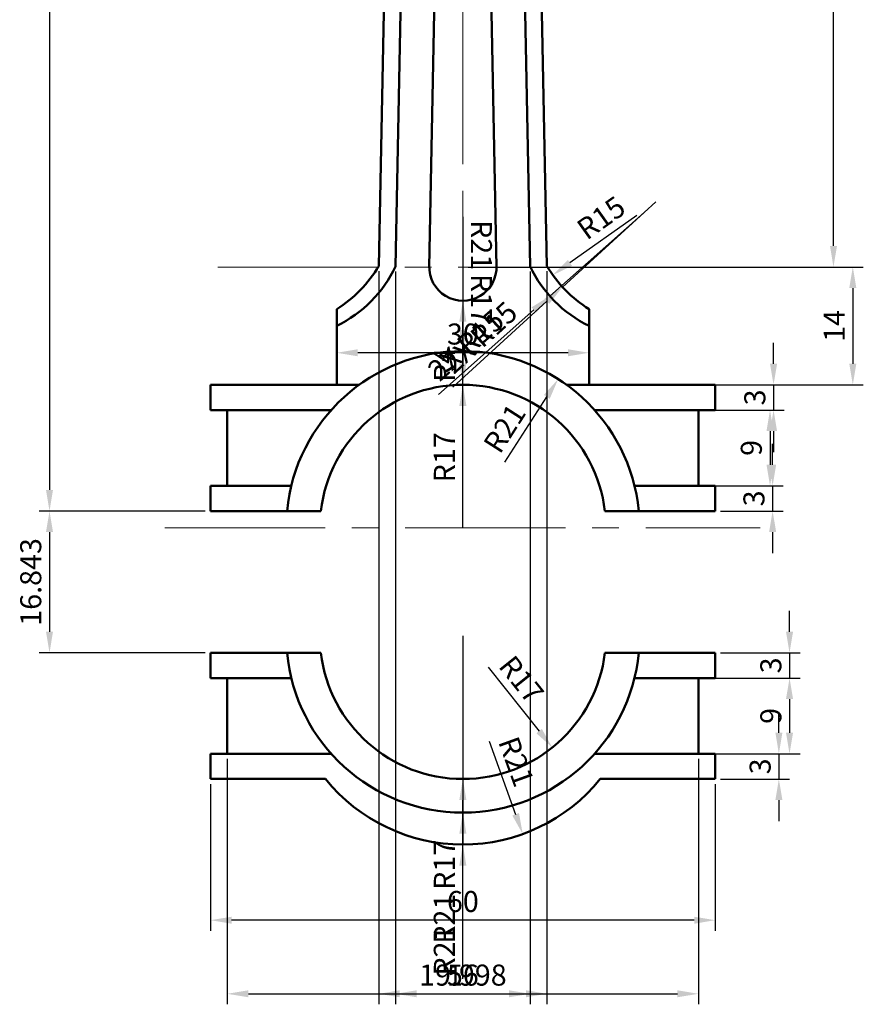
# Model space of a CAD drawing. Units: millimetres. Extents: x 2995 to 3180, y 2734 to 2968.
# Tile 1 of 3: x 2995 to 3095, y 2734 to 2851. Entities that reach past the tile are written whole.
import ezdxf

# ---------------------------------------------------------------- set-up
doc = ezdxf.new("R2010")
doc.units = ezdxf.units.MM
doc.linetypes.add('CENTER2', pattern=[28.575, 19.05, -3.175, 3.175, -3.175])
for name, color, linetype, lineweight in [('M-CNTR', 1, 'CENTER2', 18), ('M-DIMS', 2, 'Continuous', 25), ('M-OUTL', 7, 'Continuous', 50)]:
    doc.layers.add(name, color=color, linetype=linetype, lineweight=lineweight)
doc.styles.get("Standard").update_dxf_attribs({"font": 'arial.ttf'})
doc.dimstyles.new('ISO-25', dxfattribs={"dimtxt": 2.5, "dimasz": 2.5, "dimexe": 1.25, "dimexo": 0.625, "dimtad": 1, "dimtxsty": 'Standard', "dimcen": 2.5, "dimadec": 0, "dimazin": 0, "dimtfac": 1, "dimtmove": 0, "dimatfit": 3, "dimfxl": 1, "dimarcsym": 0})

# ---------------------------------------------------------------- blocks, each defined once
blk = doc.blocks.new('*D1')
at = {"layer": 'Defpoints', "color": 0, "transparency": 16777216}
for p in [(3047.54, 2807.77), (3047.54, 2790.77)]:
    blk.add_point(p, dxfattribs=at)
at = {"layer": 'M-DIMS', "color": 0, "lineweight": -2, "transparency": 16777216}
blk.add_line((3047.54, 2795.54), (3047.54, 2805.27), dxfattribs=at)
at = {"layer": 'M-DIMS', "color": 0, "transparency": 16777216}
blk.add_solid([(3047.12, 2805.27), (3047.96, 2805.27), (3047.54, 2807.77)], dxfattribs=at)
at = {"layer": 'M-DIMS', "color": 0, "transparency": 16777216, "insert": (3045.66, 2799.15), "char_height": 2.5, "attachment_point": 5, "rotation": 90}
blk.add_mtext('R17', dxfattribs=at)
blk = doc.blocks.new('*D2')
at = {"layer": 'Defpoints', "color": 0, "transparency": 16777216}
for p in [(3058.87, 2808.45), (3047.54, 2790.77)]:
    blk.add_point(p, dxfattribs=at)
at = {"layer": 'M-DIMS', "color": 0, "lineweight": -2, "transparency": 16777216}
blk.add_line((3052.53, 2798.56), (3057.52, 2806.35), dxfattribs=at)
at = {"layer": 'M-DIMS', "color": 0, "transparency": 16777216}
blk.add_solid([(3057.17, 2806.57), (3057.87, 2806.12), (3058.87, 2808.45)], dxfattribs=at)
at = {"layer": 'M-DIMS', "color": 0, "transparency": 16777216, "insert": (3052.77, 2802.42), "char_height": 2.5, "attachment_point": 5, "rotation": 57.3657}
blk.add_mtext('R21', dxfattribs=at)
blk = doc.blocks.new('*D3')
at = {"layer": 'Defpoints', "color": 0, "transparency": 16777216}
for p in [(3047.54, 2777.92), (3058.17, 2764.66)]:
    blk.add_point(p, dxfattribs=at)
at = {"layer": 'M-DIMS', "color": 0, "lineweight": -2, "transparency": 16777216}
blk.add_line((3050.53, 2774.2), (3056.61, 2766.61), dxfattribs=at)
at = {"layer": 'M-DIMS', "color": 0, "transparency": 16777216}
blk.add_solid([(3056.93, 2766.87), (3056.28, 2766.35), (3058.17, 2764.66)], dxfattribs=at)
at = {"layer": 'M-DIMS', "color": 0, "transparency": 16777216, "insert": (3054.25, 2772.55), "char_height": 2.5, "attachment_point": 5, "rotation": 308.7019}
blk.add_mtext('R17', dxfattribs=at)
blk = doc.blocks.new('*D4')
at = {"layer": 'Defpoints', "color": 0, "transparency": 16777216}
for p in [(3047.54, 2774.13), (3054.66, 2754.37)]:
    blk.add_point(p, dxfattribs=at)
at = {"layer": 'M-DIMS', "color": 0, "lineweight": -2, "transparency": 16777216}
blk.add_line((3050.68, 2765.42), (3053.81, 2756.72), dxfattribs=at)
at = {"layer": 'M-DIMS', "color": 0, "transparency": 16777216}
blk.add_solid([(3054.21, 2756.87), (3053.42, 2756.58), (3054.66, 2754.37)], dxfattribs=at)
at = {"layer": 'M-DIMS', "color": 0, "transparency": 16777216, "insert": (3053.59, 2762.88), "char_height": 2.5, "attachment_point": 5, "rotation": 289.8181}
blk.add_mtext('R21', dxfattribs=at)
blk = doc.blocks.new('*D5')
at = {"layer": 'Defpoints', "color": 0, "transparency": 16777216}
for p in [(3077.54, 2807.77), (3077.54, 2804.77), (3084.47, 2804.77)]:
    blk.add_point(p, dxfattribs=at)
at = {"layer": 'M-DIMS', "color": 0, "lineweight": -2, "transparency": 16777216}
for p, q in [((3084.47, 2810.27), (3084.47, 2812.77)), ((3078.17, 2807.77), (3085.72, 2807.77)), ((3084.47, 2807.77), (3084.47, 2804.77)), ((3078.17, 2804.77), (3085.72, 2804.77)), ((3084.47, 2802.27), (3084.47, 2799.77))]:
    blk.add_line(p, q, dxfattribs=at)
at = {"layer": 'M-DIMS', "color": 0, "transparency": 16777216}
for points in [[(3084.05, 2810.27), (3084.89, 2810.27), (3084.47, 2807.77)], [(3084.05, 2802.27), (3084.89, 2802.27), (3084.47, 2804.77)]]:
    blk.add_solid(points, dxfattribs=at)
at = {"layer": 'M-DIMS', "color": 0, "transparency": 16777216, "insert": (3082.57, 2806.27), "char_height": 2.5, "attachment_point": 5, "rotation": 90}
blk.add_mtext('3', dxfattribs=at)
blk = doc.blocks.new('*D6')
at = {"layer": 'Defpoints', "color": 0, "transparency": 16777216}
for p in [(3075.54, 2804.77), (3075.54, 2795.77), (3084.05, 2795.77)]:
    blk.add_point(p, dxfattribs=at)
at = {"layer": 'M-DIMS', "color": 0, "lineweight": -2, "transparency": 16777216}
for p, q in [((3076.17, 2804.77), (3085.3, 2804.77)), ((3084.05, 2802.27), (3084.05, 2798.27)), ((3076.17, 2795.77), (3085.3, 2795.77))]:
    blk.add_line(p, q, dxfattribs=at)
at = {"layer": 'M-DIMS', "color": 0, "transparency": 16777216}
for points in [[(3083.63, 2802.27), (3084.47, 2802.27), (3084.05, 2804.77)], [(3083.63, 2798.27), (3084.47, 2798.27), (3084.05, 2795.77)]]:
    blk.add_solid(points, dxfattribs=at)
at = {"layer": 'M-DIMS', "color": 0, "transparency": 16777216, "insert": (3082.15, 2800.27), "char_height": 2.5, "attachment_point": 5, "rotation": 90}
blk.add_mtext('9', dxfattribs=at)
blk = doc.blocks.new('*D7')
at = {"layer": 'Defpoints', "color": 0, "transparency": 16777216}
for p in [(3077.54, 2795.77), (3077.54, 2792.77), (3084.36, 2792.77)]:
    blk.add_point(p, dxfattribs=at)
at = {"layer": 'M-DIMS', "color": 0, "lineweight": -2, "transparency": 16777216}
for p, q in [((3084.36, 2798.27), (3084.36, 2800.77)), ((3078.17, 2795.77), (3085.61, 2795.77)), ((3084.36, 2795.77), (3084.36, 2792.77)), ((3078.17, 2792.77), (3085.61, 2792.77)), ((3084.36, 2790.27), (3084.36, 2787.77))]:
    blk.add_line(p, q, dxfattribs=at)
at = {"layer": 'M-DIMS', "color": 0, "transparency": 16777216}
for points in [[(3083.94, 2798.27), (3084.78, 2798.27), (3084.36, 2795.77)], [(3083.94, 2790.27), (3084.78, 2790.27), (3084.36, 2792.77)]]:
    blk.add_solid(points, dxfattribs=at)
at = {"layer": 'M-DIMS', "color": 0, "transparency": 16777216, "insert": (3082.46, 2794.27), "char_height": 2.5, "attachment_point": 5, "rotation": 90}
blk.add_mtext('3', dxfattribs=at)
blk = doc.blocks.new('*D8')
at = {"layer": 'Defpoints', "color": 0, "transparency": 16777216}
for p in [(3077.54, 2775.92), (3077.54, 2772.92), (3086.37, 2772.92)]:
    blk.add_point(p, dxfattribs=at)
at = {"layer": 'M-DIMS', "color": 0, "lineweight": -2, "transparency": 16777216}
for p, q in [((3086.37, 2778.42), (3086.37, 2780.92)), ((3078.17, 2775.92), (3087.62, 2775.92)), ((3086.37, 2775.92), (3086.37, 2772.92)), ((3078.17, 2772.92), (3087.62, 2772.92)), ((3086.37, 2770.42), (3086.37, 2767.92))]:
    blk.add_line(p, q, dxfattribs=at)
at = {"layer": 'M-DIMS', "color": 0, "transparency": 16777216}
for points in [[(3085.95, 2778.42), (3086.79, 2778.42), (3086.37, 2775.92)], [(3085.95, 2770.42), (3086.79, 2770.42), (3086.37, 2772.92)]]:
    blk.add_solid(points, dxfattribs=at)
at = {"layer": 'M-DIMS', "color": 0, "transparency": 16777216, "insert": (3084.47, 2774.42), "char_height": 2.5, "attachment_point": 5, "rotation": 90}
blk.add_mtext('3', dxfattribs=at)
blk = doc.blocks.new('*D9')
at = {"layer": 'Defpoints', "color": 0, "transparency": 16777216}
for p in [(3075.54, 2772.92), (3075.54, 2763.92), (3086.37, 2763.92)]:
    blk.add_point(p, dxfattribs=at)
at = {"layer": 'M-DIMS', "color": 0, "lineweight": -2, "transparency": 16777216}
for p, q in [((3076.17, 2772.92), (3087.62, 2772.92)), ((3086.37, 2770.42), (3086.37, 2766.42)), ((3076.17, 2763.92), (3087.62, 2763.92))]:
    blk.add_line(p, q, dxfattribs=at)
at = {"layer": 'M-DIMS', "color": 0, "transparency": 16777216}
for points in [[(3085.95, 2770.42), (3086.79, 2770.42), (3086.37, 2772.92)], [(3085.95, 2766.42), (3086.79, 2766.42), (3086.37, 2763.92)]]:
    blk.add_solid(points, dxfattribs=at)
at = {"layer": 'M-DIMS', "color": 0, "transparency": 16777216, "insert": (3084.47, 2768.42), "char_height": 2.5, "attachment_point": 5, "rotation": 90}
blk.add_mtext('9', dxfattribs=at)
blk = doc.blocks.new('*D10')
at = {"layer": 'Defpoints', "color": 0, "transparency": 16777216}
for p in [(3077.54, 2763.92), (3077.54, 2760.92), (3085.1, 2760.92)]:
    blk.add_point(p, dxfattribs=at)
at = {"layer": 'M-DIMS', "color": 0, "lineweight": -2, "transparency": 16777216}
for p, q in [((3085.1, 2766.42), (3085.1, 2768.92)), ((3078.17, 2763.92), (3086.35, 2763.92)), ((3085.1, 2763.92), (3085.1, 2760.92)), ((3078.17, 2760.92), (3086.35, 2760.92)), ((3085.1, 2758.42), (3085.1, 2755.92))]:
    blk.add_line(p, q, dxfattribs=at)
at = {"layer": 'M-DIMS', "color": 0, "transparency": 16777216}
for points in [[(3084.69, 2766.42), (3085.52, 2766.42), (3085.1, 2763.92)], [(3084.69, 2758.42), (3085.52, 2758.42), (3085.1, 2760.92)]]:
    blk.add_solid(points, dxfattribs=at)
at = {"layer": 'M-DIMS', "color": 0, "transparency": 16777216, "insert": (3083.2, 2762.42), "char_height": 2.5, "attachment_point": 5, "rotation": 90}
blk.add_mtext('3', dxfattribs=at)
blk = doc.blocks.new('*D11')
at = {"layer": 'Defpoints', "color": 0, "transparency": 16777216}
for p in [(3017.54, 2760.92), (3077.54, 2760.92), (3017.54, 2744.14)]:
    blk.add_point(p, dxfattribs=at)
at = {"layer": 'M-DIMS', "color": 0, "lineweight": -2, "transparency": 16777216}
for p, q in [((3017.54, 2760.3), (3017.54, 2742.89)), ((3077.54, 2760.3), (3077.54, 2742.89)), ((3075.04, 2744.14), (3020.04, 2744.14))]:
    blk.add_line(p, q, dxfattribs=at)
at = {"layer": 'M-DIMS', "color": 0, "transparency": 16777216}
for points in [[(3020.04, 2744.55), (3020.04, 2743.72), (3017.54, 2744.14)], [(3075.04, 2744.55), (3075.04, 2743.72), (3077.54, 2744.14)]]:
    blk.add_solid(points, dxfattribs=at)
at = {"layer": 'M-DIMS', "color": 0, "transparency": 16777216, "insert": (3047.54, 2746.04), "char_height": 2.5, "attachment_point": 5}
blk.add_mtext('60', dxfattribs=at)
blk = doc.blocks.new('*D12')
at = {"layer": 'Defpoints', "color": 0, "transparency": 16777216}
for p in [(3032.54, 2816.77), (3062.54, 2816.77), (3032.54, 2811.58)]:
    blk.add_point(p, dxfattribs=at)
at = {"layer": 'M-DIMS', "color": 0, "lineweight": -2, "transparency": 16777216}
for p, q in [((3032.54, 2816.14), (3032.54, 2810.33)), ((3062.54, 2816.14), (3062.54, 2810.33)), ((3060.04, 2811.58), (3035.04, 2811.58))]:
    blk.add_line(p, q, dxfattribs=at)
at = {"layer": 'M-DIMS', "color": 0, "transparency": 16777216}
for points in [[(3035.04, 2811.99), (3035.04, 2811.16), (3032.54, 2811.58)], [(3060.04, 2811.99), (3060.04, 2811.16), (3062.54, 2811.58)]]:
    blk.add_solid(points, dxfattribs=at)
at = {"layer": 'M-DIMS', "color": 0, "transparency": 16777216, "insert": (3047.54, 2813.48), "char_height": 2.5, "attachment_point": 5}
blk.add_mtext('30', dxfattribs=at)
blk = doc.blocks.new('*D13')
at = {"layer": 'Defpoints', "color": 0, "transparency": 16777216}
for p in [(3070.46, 2829.5), (3058.24, 2820.81)]:
    blk.add_point(p, dxfattribs=at)
at = {"layer": 'M-DIMS', "color": 0, "lineweight": -2, "transparency": 16777216}
blk.add_line((3068.21, 2827.91), (3060.27, 2822.26), dxfattribs=at)
at = {"layer": 'M-DIMS', "color": 0, "transparency": 16777216}
blk.add_solid([(3060.03, 2822.6), (3060.52, 2821.92), (3058.24, 2820.81)], dxfattribs=at)
at = {"layer": 'M-DIMS', "color": 0, "transparency": 16777216, "insert": (3064.16, 2827.36), "char_height": 2.5, "attachment_point": 5, "rotation": 35.4212}
blk.add_mtext('R15', dxfattribs=at)
blk = doc.blocks.new('*D14')
at = {"layer": 'Defpoints', "color": 0, "transparency": 16777216}
for p in [(3047.54, 2821.77), (3062.54, 2807.77), (3093.89, 2807.77)]:
    blk.add_point(p, dxfattribs=at)
at = {"layer": 'M-DIMS', "color": 0, "lineweight": -2, "transparency": 16777216}
for p, q in [((3048.17, 2821.77), (3095.14, 2821.77)), ((3093.89, 2819.27), (3093.89, 2810.27)), ((3063.17, 2807.77), (3095.14, 2807.77))]:
    blk.add_line(p, q, dxfattribs=at)
at = {"layer": 'M-DIMS', "color": 0, "transparency": 16777216}
for points in [[(3093.47, 2819.27), (3094.31, 2819.27), (3093.89, 2821.77)], [(3093.47, 2810.27), (3094.31, 2810.27), (3093.89, 2807.77)]]:
    blk.add_solid(points, dxfattribs=at)
at = {"layer": 'M-DIMS', "color": 0, "transparency": 16777216, "insert": (3092.01, 2814.77), "char_height": 2.5, "attachment_point": 5, "rotation": 90}
blk.add_mtext('14', dxfattribs=at)
blk = doc.blocks.new('*D15')
at = {"layer": 'Defpoints', "color": 0, "transparency": 16777216}
for p in [(3049.54, 2921.77), (3091.59, 2921.77), (3047.54, 2821.77)]:
    blk.add_point(p, dxfattribs=at)
at = {"layer": 'M-DIMS', "color": 0, "lineweight": -2, "transparency": 16777216}
for p, q in [((3050.17, 2921.77), (3092.84, 2921.77)), ((3091.59, 2824.27), (3091.59, 2919.27)), ((3048.17, 2821.77), (3092.84, 2821.77))]:
    blk.add_line(p, q, dxfattribs=at)
at = {"layer": 'M-DIMS', "color": 0, "transparency": 16777216}
for points in [[(3091.18, 2919.27), (3092.01, 2919.27), (3091.59, 2921.77)], [(3091.18, 2824.27), (3092.01, 2824.27), (3091.59, 2821.77)]]:
    blk.add_solid(points, dxfattribs=at)
at = {"layer": 'M-DIMS', "color": 0, "transparency": 16777216, "insert": (3089.69, 2871.77), "char_height": 2.5, "attachment_point": 5, "rotation": 90}
blk.add_mtext('100', dxfattribs=at)
blk = doc.blocks.new('*D28')
at = {"layer": 'Defpoints', "color": 0, "transparency": 16777216}
for p in [(3047.54, 2953.77), (2998.41, 2792.77), (3017.54, 2792.77)]:
    blk.add_point(p, dxfattribs=at)
at = {"layer": 'M-DIMS', "color": 0, "lineweight": -2, "transparency": 16777216}
for p, q in [((3046.92, 2953.77), (2997.16, 2953.77)), ((2998.41, 2951.27), (2998.41, 2795.27)), ((3016.92, 2792.77), (2997.16, 2792.77))]:
    blk.add_line(p, q, dxfattribs=at)
at = {"layer": 'M-DIMS', "color": 0, "transparency": 16777216}
for points in [[(2997.99, 2951.27), (2998.82, 2951.27), (2998.41, 2953.77)], [(2997.99, 2795.27), (2998.82, 2795.27), (2998.41, 2792.77)]]:
    blk.add_solid(points, dxfattribs=at)
at = {"layer": 'M-DIMS', "color": 0, "transparency": 16777216, "insert": (2996.5, 2873.27), "char_height": 2.5, "attachment_point": 5, "rotation": 90}
blk.add_mtext('161', dxfattribs=at)
blk = doc.blocks.new('*D29')
at = {"layer": 'Defpoints', "color": 0, "transparency": 16777216}
for p in [(3017.54, 2792.77), (2998.41, 2775.92), (3017.54, 2775.92)]:
    blk.add_point(p, dxfattribs=at)
at = {"layer": 'M-DIMS', "color": 0, "lineweight": -2, "transparency": 16777216}
for p, q in [((3016.92, 2792.77), (2997.16, 2792.77)), ((2998.41, 2790.27), (2998.41, 2778.42)), ((3016.92, 2775.92), (2997.16, 2775.92))]:
    blk.add_line(p, q, dxfattribs=at)
at = {"layer": 'M-DIMS', "color": 0, "transparency": 16777216}
for points in [[(2997.99, 2790.27), (2998.82, 2790.27), (2998.41, 2792.77)], [(2997.99, 2778.42), (2998.82, 2778.42), (2998.41, 2775.92)]]:
    blk.add_solid(points, dxfattribs=at)
at = {"layer": 'M-DIMS', "color": 0, "transparency": 16777216, "insert": (2996.5, 2784.34), "char_height": 2.5, "attachment_point": 5, "rotation": 90}
blk.add_mtext('16.843', dxfattribs=at)
blk = doc.blocks.new('*D32')
at = {"layer": 'Defpoints', "color": 0, "transparency": 16777216}
for p in [(3039.54, 2821.85), (3055.54, 2821.85), (3055.54, 2735.39)]:
    blk.add_point(p, dxfattribs=at)
at = {"layer": 'M-DIMS', "color": 0, "lineweight": -2, "transparency": 16777216}
for p, q in [((3039.54, 2821.22), (3039.54, 2734.14)), ((3055.54, 2821.22), (3055.54, 2734.14)), ((3042.04, 2735.39), (3053.04, 2735.39))]:
    blk.add_line(p, q, dxfattribs=at)
at = {"layer": 'M-DIMS', "color": 0, "transparency": 16777216}
for points in [[(3042.04, 2735.81), (3042.04, 2734.98), (3039.54, 2735.39)], [(3053.04, 2735.81), (3053.04, 2734.98), (3055.54, 2735.39)]]:
    blk.add_solid(points, dxfattribs=at)
at = {"layer": 'M-DIMS', "color": 0, "transparency": 16777216, "insert": (3047.54, 2737.29), "char_height": 2.5, "attachment_point": 5}
blk.add_mtext('16', dxfattribs=at)
blk = doc.blocks.new('*D33')
at = {"layer": 'Defpoints', "color": 0, "transparency": 16777216}
for p in [(3037.54, 2821.89), (3057.54, 2821.89), (3057.54, 2735.39)]:
    blk.add_point(p, dxfattribs=at)
at = {"layer": 'M-DIMS', "color": 0, "lineweight": -2, "transparency": 16777216}
for p, q in [((3037.54, 2821.26), (3037.54, 2734.14)), ((3057.54, 2821.26), (3057.54, 2734.14)), ((3040.04, 2735.39), (3055.04, 2735.39))]:
    blk.add_line(p, q, dxfattribs=at)
at = {"layer": 'M-DIMS', "color": 0, "transparency": 16777216}
for points in [[(3040.04, 2735.81), (3040.04, 2734.98), (3037.54, 2735.39)], [(3055.04, 2735.81), (3055.04, 2734.98), (3057.54, 2735.39)]]:
    blk.add_solid(points, dxfattribs=at)
at = {"layer": 'M-DIMS', "color": 0, "transparency": 16777216, "insert": (3047.54, 2737.29), "char_height": 2.5, "attachment_point": 5}
blk.add_mtext('19.998', dxfattribs=at)
blk = doc.blocks.new('*D34')
at = {"layer": 'Defpoints', "color": 0, "transparency": 16777216}
for p in [(3019.54, 2763.92), (3075.54, 2763.92), (3075.54, 2735.39)]:
    blk.add_point(p, dxfattribs=at)
at = {"layer": 'M-DIMS', "color": 0, "lineweight": -2, "transparency": 16777216}
for p, q in [((3019.54, 2763.3), (3019.54, 2734.14)), ((3075.54, 2763.3), (3075.54, 2734.14)), ((3022.04, 2735.39), (3073.04, 2735.39))]:
    blk.add_line(p, q, dxfattribs=at)
at = {"layer": 'M-DIMS', "color": 0, "transparency": 16777216}
for points in [[(3022.04, 2735.81), (3022.04, 2734.98), (3019.54, 2735.39)], [(3073.04, 2735.81), (3073.04, 2734.98), (3075.54, 2735.39)]]:
    blk.add_solid(points, dxfattribs=at)
at = {"layer": 'M-DIMS', "color": 0, "transparency": 16777216, "insert": (3047.54, 2737.29), "char_height": 2.5, "attachment_point": 5}
blk.add_mtext('56', dxfattribs=at)
blk = doc.blocks.new('*D43')
at = {"layer": 'Defpoints', "color": 0, "transparency": 16777216}
for p in [(3047.54, 2821.77), (3047.54, 2817.77)]:
    blk.add_point(p, dxfattribs=at)
at = {"layer": 'M-DIMS', "color": 0, "lineweight": -2, "transparency": 16777216}
for p, q in [((3047.54, 2821.77), (3047.54, 2817.77)), ((3047.54, 2807.5), (3047.54, 2815.27))]:
    blk.add_line(p, q, dxfattribs=at)
at = {"layer": 'M-DIMS', "color": 0, "transparency": 16777216}
blk.add_solid([(3047.12, 2815.27), (3047.96, 2815.27), (3047.54, 2817.77)], dxfattribs=at)
at = {"layer": 'M-DIMS', "color": 0, "transparency": 16777216, "insert": (3045.67, 2810.13), "char_height": 2.5, "attachment_point": 5, "rotation": 89.9963}
blk.add_mtext('R4', dxfattribs=at)
blk = doc.blocks.new('*D44')
at = {"layer": 'Defpoints', "color": 0, "transparency": 16777216}
for p in [(3070.46, 2829.5), (3059.38, 2819.39)]:
    blk.add_point(p, dxfattribs=at)
at = {"layer": 'M-DIMS', "color": 0, "lineweight": -2, "transparency": 16777216}
for p, q in [((3070.46, 2829.5), (3059.38, 2819.39)), ((3046.34, 2807.49), (3057.54, 2817.71))]:
    blk.add_line(p, q, dxfattribs=at)
at = {"layer": 'M-DIMS', "color": 0, "transparency": 16777216}
blk.add_solid([(3057.25, 2818.01), (3057.82, 2817.4), (3059.38, 2819.39)], dxfattribs=at)
at = {"layer": 'M-DIMS', "color": 0, "transparency": 16777216, "insert": (3049.73, 2813.16), "char_height": 2.5, "attachment_point": 5, "rotation": 42.3887}
blk.add_mtext('2X R15', dxfattribs=at)
blk = doc.blocks.new('*D45')
at = {"layer": 'Defpoints', "color": 0, "transparency": 16777216}
for p in [(3069.1, 2828.26), (3057.86, 2818.32)]:
    blk.add_point(p, dxfattribs=at)
at = {"layer": 'M-DIMS', "color": 0, "lineweight": -2, "transparency": 16777216}
for p, q in [((3069.1, 2828.26), (3057.86, 2818.32)), ((3044.63, 2806.63), (3055.99, 2816.67))]:
    blk.add_line(p, q, dxfattribs=at)
at = {"layer": 'M-DIMS', "color": 0, "transparency": 16777216}
blk.add_solid([(3055.71, 2816.98), (3056.27, 2816.35), (3057.86, 2818.32)], dxfattribs=at)
at = {"layer": 'M-DIMS', "color": 0, "transparency": 16777216, "insert": (3048.12, 2812.24), "char_height": 2.5, "attachment_point": 5, "rotation": 41.473}
blk.add_mtext('2X R15', dxfattribs=at)
blk = doc.blocks.new('*D46')
at = {"layer": 'Defpoints', "color": 0, "transparency": 16777216}
for p in [(3047.54, 2811.77), (3047.54, 2790.77)]:
    blk.add_point(p, dxfattribs=at)
at = {"layer": 'M-DIMS', "color": 0, "lineweight": -2, "transparency": 16777216}
for p, q in [((3047.54, 2827.74), (3047.54, 2814.27)), ((3047.54, 2790.77), (3047.54, 2811.77))]:
    blk.add_line(p, q, dxfattribs=at)
at = {"layer": 'M-DIMS', "color": 0, "transparency": 16777216}
blk.add_solid([(3047.96, 2814.27), (3047.12, 2814.27), (3047.54, 2811.77)], dxfattribs=at)
at = {"layer": 'M-DIMS', "color": 0, "transparency": 16777216, "insert": (3049.42, 2824.37), "char_height": 2.5, "attachment_point": 5, "rotation": 270.0007}
blk.add_mtext('R21', dxfattribs=at)
blk = doc.blocks.new('*D47')
at = {"layer": 'Defpoints', "color": 0, "transparency": 16777216}
for p in [(3047.54, 2807.77), (3047.54, 2790.77)]:
    blk.add_point(p, dxfattribs=at)
at = {"layer": 'M-DIMS', "color": 0, "lineweight": -2, "transparency": 16777216}
for p, q in [((3047.54, 2821.58), (3047.54, 2810.27)), ((3047.54, 2790.77), (3047.54, 2807.77))]:
    blk.add_line(p, q, dxfattribs=at)
at = {"layer": 'M-DIMS', "color": 0, "transparency": 16777216}
blk.add_solid([(3047.96, 2810.27), (3047.12, 2810.27), (3047.54, 2807.77)], dxfattribs=at)
at = {"layer": 'M-DIMS', "color": 0, "transparency": 16777216, "insert": (3049.42, 2817.97), "char_height": 2.5, "attachment_point": 5, "rotation": 270.0009}
blk.add_mtext('R17', dxfattribs=at)
blk = doc.blocks.new('*D48')
at = {"layer": 'Defpoints', "color": 0, "transparency": 16777216}
for p in [(3047.54, 2777.92), (3047.54, 2760.92)]:
    blk.add_point(p, dxfattribs=at)
at = {"layer": 'M-DIMS', "color": 0, "lineweight": -2, "transparency": 16777216}
for p, q in [((3047.54, 2777.92), (3047.54, 2760.92)), ((3047.54, 2747.11), (3047.54, 2758.42))]:
    blk.add_line(p, q, dxfattribs=at)
at = {"layer": 'M-DIMS', "color": 0, "transparency": 16777216}
blk.add_solid([(3047.12, 2758.42), (3047.96, 2758.42), (3047.54, 2760.92)], dxfattribs=at)
at = {"layer": 'M-DIMS', "color": 0, "transparency": 16777216, "insert": (3045.66, 2750.72), "char_height": 2.5, "attachment_point": 5, "rotation": 89.9991}
blk.add_mtext('R17', dxfattribs=at)
blk = doc.blocks.new('*D49')
at = {"layer": 'Defpoints', "color": 0, "transparency": 16777216}
for p in [(3047.54, 2777.92), (3047.54, 2756.92)]:
    blk.add_point(p, dxfattribs=at)
at = {"layer": 'M-DIMS', "color": 0, "lineweight": -2, "transparency": 16777216}
for p, q in [((3047.54, 2777.92), (3047.54, 2756.92)), ((3047.54, 2740.95), (3047.54, 2754.42))]:
    blk.add_line(p, q, dxfattribs=at)
at = {"layer": 'M-DIMS', "color": 0, "transparency": 16777216}
blk.add_solid([(3047.12, 2754.42), (3047.96, 2754.42), (3047.54, 2756.92)], dxfattribs=at)
at = {"layer": 'M-DIMS', "color": 0, "transparency": 16777216, "insert": (3045.66, 2744.32), "char_height": 2.5, "attachment_point": 5, "rotation": 89.9993}
blk.add_mtext('R21', dxfattribs=at)
blk = doc.blocks.new('*D50')
at = {"layer": 'Defpoints', "color": 0, "transparency": 16777216}
for p in [(3047.54, 2774.13), (3047.54, 2753.13)]:
    blk.add_point(p, dxfattribs=at)
at = {"layer": 'M-DIMS', "color": 0, "lineweight": -2, "transparency": 16777216}
for p, q in [((3047.54, 2774.13), (3047.54, 2753.13)), ((3047.54, 2737.16), (3047.54, 2750.63))]:
    blk.add_line(p, q, dxfattribs=at)
at = {"layer": 'M-DIMS', "color": 0, "transparency": 16777216}
blk.add_solid([(3047.12, 2750.63), (3047.96, 2750.63), (3047.54, 2753.13)], dxfattribs=at)
at = {"layer": 'M-DIMS', "color": 0, "transparency": 16777216, "insert": (3045.66, 2740.53), "char_height": 2.5, "attachment_point": 5, "rotation": 89.9993}
blk.add_mtext('R21', dxfattribs=at)

msp = doc.modelspace()

# ---------------------------------------------------------------- linework, layer by layer
at = {"layer": 'M-CNTR'}
for p, q in [((3047.5413, 2938.7662), (3047.5413, 2821.7662)), ((3018.4256, 2821.7662), (3087.998, 2821.7662)), ((3047.5413, 2821.7662), (3047.5413, 2814.7662)), ((3047.5413, 2807.7662), (3047.5413, 2790.7662)), ((3012.1191, 2790.7662), (3082.8947, 2790.7662)), ((3047.5413, 2760.9236), (3047.5413, 2777.9236))]:
    msp.add_line(p, q, dxfattribs=at)
at = {"layer": 'M-OUTL'}
for p, q in [((3041.5351, 2921.4996), (3039.5421, 2821.8462)), ((3045.5413, 2921.7662), (3043.5413, 2821.7662)), ((3049.5413, 2921.7662), (3051.5413, 2821.7662)), ((3053.5474, 2921.4996), (3055.5405, 2821.8462)), ((3039.49, 2919.2627), (3037.5425, 2821.8862)), ((3055.5925, 2919.2627), (3057.5401, 2821.8862)), ((3032.5413, 2814.7662), (3032.5413, 2816.7662)), ((3062.5413, 2814.7662), (3062.5413, 2816.7662)), ((3032.5413, 2814.7662), (3032.5413, 2807.7662)), ((3062.5413, 2814.7662), (3062.5413, 2807.7662)), ((3017.5413, 2804.7662), (3017.5413, 2807.7662)), ((3017.5413, 2807.7662), (3032.5413, 2807.7662)), ((3035.2124, 2807.7662), (3032.5413, 2807.7662)), ((3062.5413, 2807.7662), (3059.8701, 2807.7662)), ((3062.5413, 2807.7662), (3077.5413, 2807.7662)), ((3077.5413, 2807.7662), (3077.5413, 2804.7662)), ((3031.8888, 2804.7662), (3017.5413, 2804.7662)), ((3019.5413, 2804.7662), (3017.5413, 2804.7662)), ((3019.5413, 2795.7662), (3019.5413, 2804.7662)), ((3077.5413, 2804.7662), (3063.1937, 2804.7662)), ((3077.5413, 2804.7662), (3075.5413, 2804.7662)), ((3075.5413, 2804.7662), (3075.5413, 2795.7662)), ((3017.5413, 2792.7662), (3017.5413, 2795.7662)), ((3017.5413, 2795.7662), (3019.5413, 2795.7662)), ((3027.1452, 2795.7662), (3019.5413, 2795.7662)), ((3075.5413, 2795.7662), (3067.9373, 2795.7662)), ((3075.5413, 2795.7662), (3077.5413, 2795.7662)), ((3077.5413, 2795.7662), (3077.5413, 2792.7662)), ((3026.6367, 2792.7662), (3017.5413, 2792.7662)), ((3026.6367, 2792.7662), (3030.6593, 2792.7662)), ((3064.4232, 2792.7662), (3068.4458, 2792.7662)), ((3077.5413, 2792.7662), (3068.4458, 2792.7662)), ((3017.5413, 2772.9236), (3017.5413, 2775.9236)), ((3017.5413, 2775.9236), (3026.6367, 2775.9236)), ((3030.6593, 2775.9236), (3026.6367, 2775.9236)), ((3068.4458, 2775.9236), (3064.4232, 2775.9236)), ((3068.4458, 2775.9236), (3077.5413, 2775.9236)), ((3077.5413, 2775.9236), (3077.5413, 2772.9236)), ((3019.5413, 2772.9236), (3017.5413, 2772.9236)), ((3019.5413, 2763.9236), (3019.5413, 2772.9236)), ((3019.5413, 2772.9236), (3027.1452, 2772.9236)), ((3067.9373, 2772.9236), (3075.5413, 2772.9236)), ((3075.5413, 2772.9236), (3075.5413, 2763.9236)), ((3077.5413, 2772.9236), (3075.5413, 2772.9236)), ((3017.5413, 2760.9236), (3017.5413, 2763.9236)), ((3017.5413, 2763.9236), (3031.8888, 2763.9236)), ((3017.5413, 2763.9236), (3019.5413, 2763.9236)), ((3063.1937, 2763.9236), (3077.5413, 2763.9236)), ((3075.5413, 2763.9236), (3077.5413, 2763.9236)), ((3077.5413, 2763.9236), (3077.5413, 2760.9236)), ((3031.2124, 2760.9236), (3017.5413, 2760.9236)), ((3077.5413, 2760.9236), (3063.8701, 2760.9236))]:
    msp.add_line(p, q, dxfattribs=at)
for centre, radius, start, end in [((3024.6214, 2829.5049), 15, 301.869919, 329.4748), ((3025.9802, 2828.2552), 15, 295.93852, 334.705886), ((3047.5413, 2821.7662), 4, 177.708474, 2.291526), ((3069.1024, 2828.2552), 15, 205.294114, 244.06148), ((3070.4611, 2829.5049), 15, 210.5252, 238.130081), ((3047.5413, 2790.7662), 21, 5.465024, 174.534976), ((3047.5413, 2790.7662), 17, 6.756327, 173.243673), ((3047.5413, 2777.9236), 21, 185.465024, 354.534976), ((3047.5413, 2777.9236), 17, 186.756327, 353.243673), ((3047.5413, 2774.1285), 21, 218.961994, 321.038006)]:
    msp.add_arc(centre, radius, start, end, dxfattribs=at)

# ---------------------------------------------------------------- dimensions: what is measured, and where the dimension line sits
at = {"layer": 'M-DIMS'}
for base, p1, p2, override, picture, middle in [((2998.4052, 2792.7662), (3047.5413, 2953.7662), (3017.5413, 2792.7662), {"dimdec": 0, "dimlfac": 1, "dimrnd": 0, "dimzin": 0, "dimdsep": 46, "dimlunit": 2}, '*D28', (2996.5038, 2873.2662)), ((3091.5923, 2921.7662), (3047.5413, 2821.7662), (3049.5413, 2921.7662), {"dimclrd": 0, "dimclre": 0, "dimclrt": 0}, '*D15', (3089.6908, 2871.7662)), ((3093.8887, 2807.7662), (3047.5413, 2821.7662), (3062.5413, 2807.7662), {"dimclrd": 0, "dimclre": 0, "dimclrt": 0}, '*D14', (3092.0086, 2814.7662)), ((3084.4716, 2804.7662), (3077.5413, 2807.7662), (3077.5413, 2804.7662), {"dimclrd": 0, "dimclre": 0, "dimclrt": 0}, '*D5', (3082.5693, 2806.2662)), ((3084.0497, 2795.7662), (3075.5413, 2804.7662), (3075.5413, 2795.7662), {"dimclrd": 0, "dimclre": 0, "dimclrt": 0}, '*D6', (3082.1483, 2800.2662)), ((3084.3603, 2792.7662), (3077.5413, 2795.7662), (3077.5413, 2792.7662), {"dimclrd": 0, "dimclre": 0, "dimclrt": 0}, '*D7', (3082.458, 2794.2662)), ((2998.4052, 2775.9236), (3017.5413, 2792.7662), (3017.5413, 2775.9236), {"dimdec": 3, "dimlfac": 1, "dimrnd": 0, "dimzin": 0, "dimdsep": 46, "dimlunit": 2}, '*D29', (2996.5029, 2784.3449)), ((3086.3701, 2772.9236), (3077.5413, 2775.9236), (3077.5413, 2772.9236), {"dimclrd": 0, "dimclre": 0, "dimclrt": 0}, '*D8', (3084.4678, 2774.4236)), ((3086.3701, 2763.9236), (3075.5413, 2772.9236), (3075.5413, 2763.9236), {"dimclrd": 0, "dimclre": 0, "dimclrt": 0}, '*D9', (3084.4686, 2768.4236)), ((3085.1044, 2760.9236), (3077.5413, 2763.9236), (3077.5413, 2760.9236), {"dimclrd": 0, "dimclre": 0, "dimclrt": 0}, '*D10', (3083.2021, 2762.4236))]:
    dim = msp.add_linear_dim(base=base, p1=p1, p2=p2, angle=90, dimstyle='ISO-25', override=override, dxfattribs=at)
    dim.commit()
    dim.dimension.update_dxf_attribs({"geometry": picture, "text_midpoint": middle})
for center, mpoint, override, picture, middle in [((3070.4611, 2829.5049), (3058.2374, 2820.8112), {"dimclrd": 0, "dimclre": 0, "dimclrt": 0}, '*D13', (3065.263, 2825.8079)), ((3047.5413, 2790.7662), (3047.541, 2811.7662), {"dimdec": 0, "dimlfac": 1, "dimrnd": 0, "dimzin": 0, "dimdsep": 46, "dimlunit": 2}, '*D46', (3047.5408, 2824.3662)), ((3047.5413, 2790.7662), (3047.541, 2807.7662), {"dimdec": 0, "dimlfac": 1, "dimrnd": 0, "dimzin": 0, "dimdsep": 46, "dimlunit": 2}, '*D47', (3047.5408, 2817.9662)), ((3047.5413, 2790.7662), (3047.5413, 2807.7662), {"dimclrd": 0, "dimclre": 0, "dimclrt": 0}, '*D1', (3047.5413, 2799.1543)), ((3047.5413, 2790.7662), (3058.866, 2808.4509), {"dimclrd": 0, "dimclre": 0, "dimclrt": 0}, '*D2', (3054.352, 2801.4018)), ((3047.5413, 2777.9236), (3047.541, 2760.9236), {"dimdec": 0, "dimlfac": 1, "dimrnd": 0, "dimzin": 0, "dimdsep": 46, "dimlunit": 2}, '*D48', (3047.5408, 2750.7236)), ((3047.5413, 2777.9236), (3047.541, 2756.9236), {"dimdec": 0, "dimlfac": 1, "dimrnd": 0, "dimzin": 0, "dimdsep": 46, "dimlunit": 2}, '*D49', (3047.5408, 2744.3236)), ((3047.5413, 2777.9236), (3058.1708, 2764.6567), {"dimclrd": 0, "dimclre": 0, "dimclrt": 0}, '*D3', (3052.7861, 2771.3774)), ((3047.5413, 2774.1285), (3047.541, 2753.1285), {"dimdec": 0, "dimlfac": 1, "dimrnd": 0, "dimzin": 0, "dimdsep": 46, "dimlunit": 2}, '*D50', (3047.5408, 2740.5285)), ((3047.5413, 2774.1285), (3054.661, 2754.3723), {"dimclrd": 0, "dimclre": 0, "dimclrt": 0}, '*D4', (3051.8231, 2762.2471))]:
    dim = msp.add_radius_dim(center=center, mpoint=mpoint, dimstyle='ISO-25', override=override, dxfattribs=at)
    dim.commit()
    dim.dimension.update_dxf_attribs({"geometry": picture, "text_midpoint": middle, "dimtype": 164})
for center, mpoint, picture, middle in [((3070.4611, 2829.5049), (3059.3823, 2819.3926), '*D44', (3049.7334, 2813.1598)), ((3069.1024, 2828.2552), (3057.8633, 2818.3211), '*D45', (3048.116, 2812.2434))]:
    dim = msp.add_radius_dim(center=center, mpoint=mpoint, text='2X <>', dimstyle='ISO-25', override={"dimdec": 0, "dimlfac": 1, "dimrnd": 0, "dimzin": 0, "dimdsep": 46, "dimlunit": 2}, dxfattribs=at)
    dim.commit()
    dim.dimension.update_dxf_attribs({"geometry": picture, "text_midpoint": middle})
for base, p1, p2, override, picture, middle in [((3057.5401, 2735.3926), (3037.5425, 2821.8862), (3057.5401, 2821.8862), {"dimdec": 3, "dimlfac": 1, "dimrnd": 0, "dimzin": 0, "dimdsep": 46, "dimlunit": 2}, '*D33', (3047.5413, 2737.2941)), ((3055.5405, 2735.3926), (3039.5421, 2821.8462), (3055.5405, 2821.8462), {"dimdec": 0, "dimlfac": 1, "dimrnd": 0, "dimzin": 0, "dimdsep": 46, "dimlunit": 2}, '*D32', (3047.5413, 2737.2941)), ((3032.5413, 2811.5777), (3062.5413, 2816.7662), (3032.5413, 2816.7662), {"dimclrd": 0, "dimclre": 0, "dimclrt": 0}, '*D12', (3047.5413, 2813.48)), ((3075.5413, 2735.3926), (3019.5413, 2763.9236), (3075.5413, 2763.9236), {"dimdec": 0, "dimlfac": 1, "dimrnd": 0, "dimzin": 0, "dimdsep": 46, "dimlunit": 2}, '*D34', (3047.5413, 2737.2941)), ((3017.5413, 2744.1363), (3077.5413, 2760.9236), (3017.5413, 2760.9236), {"dimclrd": 0, "dimclre": 0, "dimclrt": 0}, '*D11', (3047.5413, 2746.0377))]:
    dim = msp.add_linear_dim(base=base, p1=p1, p2=p2, dimstyle='ISO-25', override=override, dxfattribs=at)
    dim.commit()
    dim.dimension.update_dxf_attribs({"geometry": picture, "text_midpoint": middle})
dim = msp.add_radius_dim(center=(3047.5413, 2821.7662), mpoint=(3047.541, 2817.7662), dimstyle='ISO-25', override={"dimdec": 0, "dimlfac": 1, "dimrnd": 0, "dimzin": 0, "dimdsep": 46, "dimlunit": 2}, dxfattribs=at)
dim.commit()
dim.dimension.update_dxf_attribs({"geometry": '*D43', "text_midpoint": (3045.6655, 2810.1307)})

doc.saveas('drawing.dxf')
